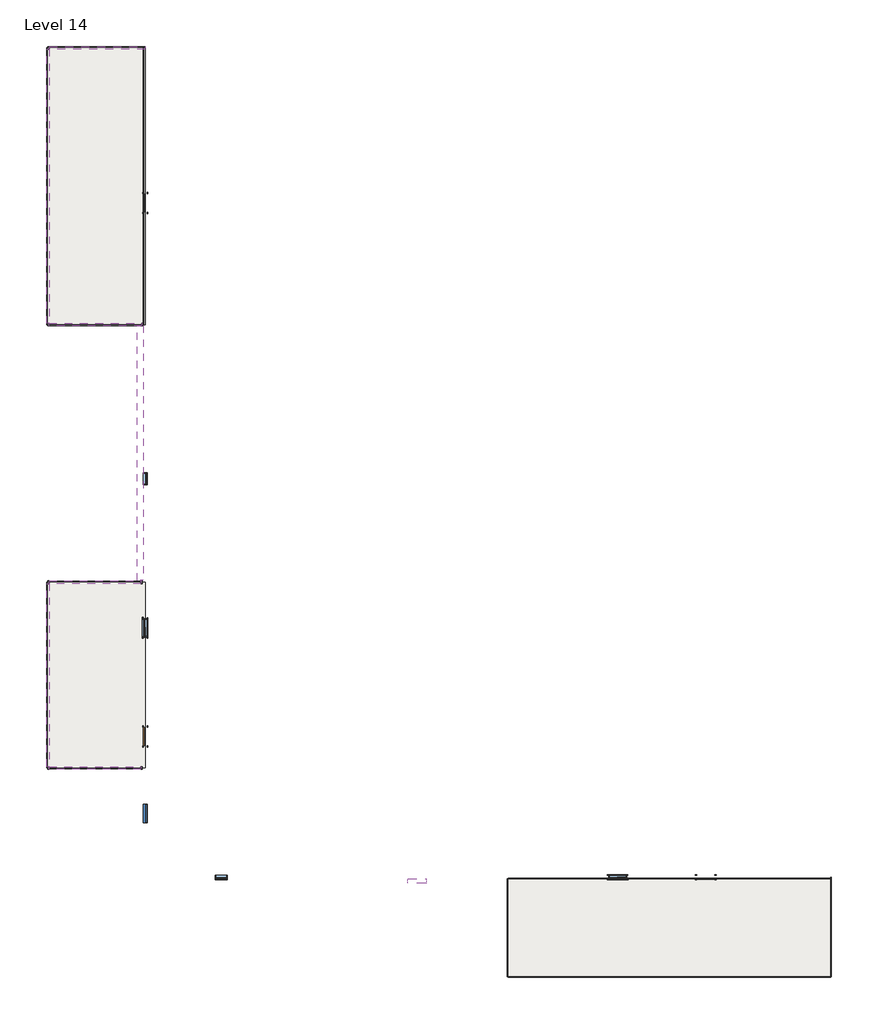
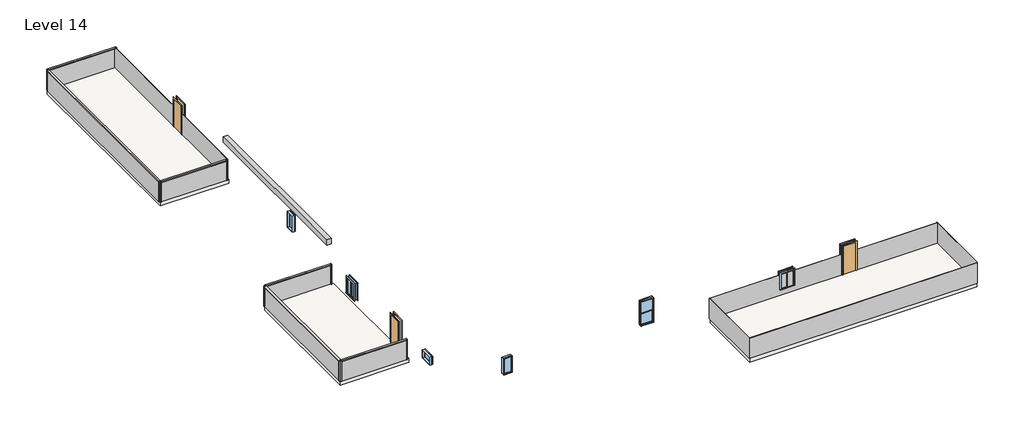
# One storey: 17 members, 11 plates, 6 windows, 3 doors, 3 slabs, 1 proxy.
"""IFC4 building model written with IfcOpenShell, lengths in millimetres."""

from ifc_helpers import new_model, si_unit, frame, origin, place, context, project, spatial, polyline, outline, extrude, transform, mapped, element, save
from components import generic_models_16_generic_models_16_858d129d, door_54dd4da4, door_719f80de, member_a0ba9e48, member_4491d118, member_315671ef, member_43964152, member_8787ee90, member_2afbfae4, system_panel_glazed_dbf8c7ac, system_panel_glazed_64af9de3, system_panel_glazed_abcfc967, system_panel_glazed_48350550, system_panel_glazed_82bc3a22, system_panel_glazed_a411ffd8, system_panel_glazed_b08a8197, system_panel_glazed_fce9463a, system_panel_glazed_627c678d, window_f274a882, window_80bd9af0, window_57c3ee1c, window_78885257, window_54100e87

model = new_model("IFC4")

# Units and contexts
model_context = context("Model", 3, world=origin())
ifc_project = project(units=[si_unit("LENGTHUNIT", "METRE", prefix="MILLI")], contexts=[model_context])

# Site, building, storey
site = spatial("IfcSite", under=ifc_project)
building = spatial("IfcBuilding", under=site)
storey = spatial("IfcBuildingStorey", under=building, Name="Level 14", Elevation=23164.8)

# Proxy
placement = place(None, origin())
generic_models_16_generic_models_16_shape = generic_models_16_generic_models_16_858d129d(model_context)
element("IfcBuildingElementProxy", 1, Name="Generic Models 16 : Generic Models 16", ObjectType="Generic Models 16 : Generic Models 16", at=placement, inside=storey, context=model_context, shape_type="MappedRepresentation", body=[
    mapped(generic_models_16_generic_models_16_shape, transform((0.0, 0.0, 0.0), x_axis=(1.0, 0.0, 0.0), y_axis=(0.0, 1.0, 0.0), z_axis=(0.0, 0.0, 1.0))),
])

# Doors
door_shape = door_54dd4da4(model_context)
element("IfcDoor", 2, ObjectType="Single-Flush : 36\" x 84\"", at=placement, inside=storey, context=model_context, shape_type="MappedRepresentation", body=[
    mapped(door_shape, transform((-15175.038074, 13037.8014639, 23164.8), x_axis=(0.0, 1.0, 0.0), y_axis=(-1.0, 0.0, 0.0), z_axis=(0.0, 0.0, 1.0))),
])
element("IfcDoor", 3, ObjectType="Single-Flush : 36\" x 84\"", at=placement, inside=storey, context=model_context, shape_type="MappedRepresentation", body=[
    mapped(door_shape, transform((-15175.038074, -13700.1915889, 23164.8), x_axis=(0.0, 1.0, 0.0), y_axis=(-1.0, 0.0, 0.0), z_axis=(0.0, 0.0, 1.0))),
])
door_2_shape = door_719f80de(model_context)
element("IfcDoor", 4, ObjectType="Single-Flush : 36\" x 84\"", at=placement, inside=storey, context=model_context, shape_type="MappedRepresentation", body=[
    mapped(door_2_shape, transform((12917.361926, -20744.1985361, 23164.8), x_axis=(1.0, 0.0, 0.0), y_axis=(0.0, 1.0, 0.0), z_axis=(0.0, 0.0, 1.0))),
])

# Members
member_shape = member_a0ba9e48(model_context)
element("IfcMember", 5, ObjectType="Rectangular Mullion : 2.5\" x 5\" rectangular", at=placement, inside=storey, context=model_context, shape_type="MappedRepresentation", body=[
    mapped(member_shape, transform((-15175.038074, 20810.2014639, 24688.8), x_axis=(0.0, 0.0, 1.0), y_axis=(0.0, -1.0, 0.0), z_axis=(1.0, 0.0, 0.0))),
])
member_2_shape = member_4491d118(model_context)
element("IfcMember", 6, ObjectType="Rectangular Mullion : 2.5\" x 5\" rectangular", at=placement, inside=storey, context=model_context, shape_type="MappedRepresentation", body=[
    mapped(member_2_shape, transform((-20051.838074, 6941.8014639, 23164.8), x_axis=(-1.0, 0.0, 0.0), y_axis=(0.0, 1.0, 0.0), z_axis=(0.0, 0.0, -1.0))),
])
element("IfcMember", 7, ObjectType="Rectangular Mullion : 2.5\" x 5\" rectangular", at=placement, inside=storey, context=model_context, shape_type="MappedRepresentation", body=[
    mapped(member_2_shape, transform((-20051.838074, 20810.2014639, 23164.8), x_axis=(0.0, 1.0, 0.0), y_axis=(1.0, 0.0, 0.0), z_axis=(0.0, 0.0, -1.0))),
])
element("IfcMember", 8, ObjectType="Rectangular Mullion : 2.5\" x 5\" rectangular", at=placement, inside=storey, context=model_context, shape_type="MappedRepresentation", body=[
    mapped(member_2_shape, transform((-20051.838074, -15263.2213044, 23164.8), x_axis=(-1.0, 0.0, 0.0), y_axis=(0.0, 1.0, 0.0), z_axis=(0.0, 0.0, -1.0))),
])
element("IfcMember", 9, ObjectType="Rectangular Mullion : 2.5\" x 5\" rectangular", at=placement, inside=storey, context=model_context, shape_type="MappedRepresentation", body=[
    mapped(member_2_shape, transform((-20051.838074, -5966.8213044, 23164.8), x_axis=(0.0, 1.0, 0.0), y_axis=(1.0, 0.0, 0.0), z_axis=(0.0, 0.0, -1.0))),
])
element("IfcMember", 10, ObjectType="Rectangular Mullion : 2.5\" x 5\" rectangular", at=placement, inside=storey, context=model_context, shape_type="MappedRepresentation", body=[
    mapped(member_2_shape, transform((-15319.7124518, -5966.8213044, 23164.8), x_axis=(1.0, 0.0, 0.0), y_axis=(0.0, -1.0, 0.0), z_axis=(0.0, 0.0, -1.0))),
])
element("IfcMember", 11, ObjectType="Rectangular Mullion : 2.5\" x 5\" rectangular", at=placement, inside=storey, context=model_context, shape_type="MappedRepresentation", body=[
    mapped(member_2_shape, transform((-20051.838074, 6941.8014639, 24688.8), x_axis=(0.0, -1.0, 0.0), y_axis=(1.0, 0.0, 0.0), z_axis=(0.0, 0.0, 1.0))),
])
element("IfcMember", 12, ObjectType="Rectangular Mullion : 2.5\" x 5\" rectangular", at=placement, inside=storey, context=model_context, shape_type="MappedRepresentation", body=[
    mapped(member_2_shape, transform((-15282.7172704, 6941.8014639, 24688.8), x_axis=(1.0, 0.0, 0.0), y_axis=(0.0, 1.0, 0.0), z_axis=(0.0, 0.0, 1.0))),
])
element("IfcMember", 13, ObjectType="Rectangular Mullion : 2.5\" x 5\" rectangular", at=placement, inside=storey, context=model_context, shape_type="MappedRepresentation", body=[
    mapped(member_2_shape, transform((-20051.838074, 20810.2014639, 24688.8), x_axis=(-1.0, 0.0, 0.0), y_axis=(0.0, -1.0, 0.0), z_axis=(0.0, 0.0, 1.0))),
])
element("IfcMember", 14, ObjectType="Rectangular Mullion : 2.5\" x 5\" rectangular", at=placement, inside=storey, context=model_context, shape_type="MappedRepresentation", body=[
    mapped(member_2_shape, transform((-20051.838074, -15263.2213044, 24688.8), x_axis=(0.0, -1.0, 0.0), y_axis=(1.0, 0.0, 0.0), z_axis=(0.0, 0.0, 1.0))),
])
element("IfcMember", 15, ObjectType="Rectangular Mullion : 2.5\" x 5\" rectangular", at=placement, inside=storey, context=model_context, shape_type="MappedRepresentation", body=[
    mapped(member_2_shape, transform((-15319.7124518, -15263.2213044, 24688.8), x_axis=(1.0, 0.0, 0.0), y_axis=(0.0, 1.0, 0.0), z_axis=(0.0, 0.0, 1.0))),
])
element("IfcMember", 16, ObjectType="Rectangular Mullion : 2.5\" x 5\" rectangular", at=placement, inside=storey, context=model_context, shape_type="MappedRepresentation", body=[
    mapped(member_2_shape, transform((-20051.838074, -5966.8213044, 24688.8), x_axis=(-1.0, 0.0, 0.0), y_axis=(0.0, -1.0, 0.0), z_axis=(0.0, 0.0, 1.0))),
])
member_3_shape = member_315671ef(model_context)
element("IfcMember", 17, ObjectType="Rectangular Mullion : 2.5\" x 5\" rectangular", at=placement, inside=storey, context=model_context, shape_type="MappedRepresentation", body=[
    mapped(member_3_shape, transform((-20051.838074, 20746.7014639, 24688.8), x_axis=(0.0, 0.0, 1.0), y_axis=(1.0, 0.0, 0.0), z_axis=(0.0, 1.0, 0.0))),
])
member_4_shape = member_43964152(model_context)
element("IfcMember", 18, ObjectType="Rectangular Mullion : 2.5\" x 5\" rectangular", at=placement, inside=storey, context=model_context, shape_type="MappedRepresentation", body=[
    mapped(member_4_shape, transform((-19988.338074, 6941.8014639, 24688.8), x_axis=(0.0, 0.0, 1.0), y_axis=(0.0, 1.0, 0.0), z_axis=(-1.0, 0.0, 0.0))),
])
member_5_shape = member_8787ee90(model_context)
element("IfcMember", 19, ObjectType="Rectangular Mullion : 2.5\" x 5\" rectangular", at=placement, inside=storey, context=model_context, shape_type="MappedRepresentation", body=[
    mapped(member_5_shape, transform((-20051.838074, -6030.3213044, 24688.8), x_axis=(0.0, 0.0, 1.0), y_axis=(1.0, 0.0, 0.0), z_axis=(0.0, 1.0, 0.0))),
])
member_6_shape = member_2afbfae4(model_context)
element("IfcMember", 20, ObjectType="Rectangular Mullion : 2.5\" x 5\" rectangular", at=placement, inside=storey, context=model_context, shape_type="MappedRepresentation", body=[
    mapped(member_6_shape, transform((-19988.338074, -15263.2213044, 24688.8), x_axis=(0.0, 0.0, 1.0), y_axis=(0.0, 1.0, 0.0), z_axis=(-1.0, 0.0, 0.0))),
])
element("IfcMember", 21, ObjectType="Rectangular Mullion : 2.5\" x 5\" rectangular", at=placement, inside=storey, context=model_context, shape_type="MappedRepresentation", body=[
    mapped(member_6_shape, transform((-15383.2124518, -5966.8213044, 24688.8), x_axis=(0.0, 0.0, 1.0), y_axis=(0.0, -1.0, 0.0), z_axis=(1.0, 0.0, 0.0))),
])

# Plates
system_panel_glazed_shape = system_panel_glazed_dbf8c7ac(model_context)
element("IfcPlate", 22, ObjectType="System Panel : Glazed", at=placement, inside=storey, context=model_context, shape_type="MappedRepresentation", body=[
    mapped(system_panel_glazed_shape, transform((11088.561926, -20845.7985361, 23164.8), x_axis=(1.0, 0.0, 0.0), y_axis=(0.0, 1.0, 0.0), z_axis=(0.0, 0.0, 1.0))),
])
element("IfcPlate", 23, ObjectType="System Panel : Glazed", at=placement, inside=storey, context=model_context, shape_type="MappedRepresentation", body=[
    mapped(system_panel_glazed_shape, transform((11088.561926, -25722.5985361, 23164.8), x_axis=(-1.0, 0.0, 0.0), y_axis=(0.0, -1.0, 0.0), z_axis=(0.0, 0.0, 1.0))),
])
system_panel_glazed_2_shape = system_panel_glazed_64af9de3(model_context)
element("IfcPlate", 24, ObjectType="System Panel : Glazed", at=placement, inside=storey, context=model_context, shape_type="MappedRepresentation", body=[
    mapped(system_panel_glazed_2_shape, transform((19165.761926, -23233.3985361, 23164.8), x_axis=(0.0, -1.0, 0.0), y_axis=(1.0, 0.0, 0.0), z_axis=(0.0, 0.0, 1.0))),
])
system_panel_glazed_3_shape = system_panel_glazed_abcfc967(model_context)
element("IfcPlate", 25, ObjectType="System Panel : Glazed", at=placement, inside=storey, context=model_context, shape_type="MappedRepresentation", body=[
    mapped(system_panel_glazed_3_shape, transform((3011.361926, -23273.4060583, 23164.8), x_axis=(0.0, 1.0, 0.0), y_axis=(-1.0, 0.0, 0.0), z_axis=(0.0, 0.0, 1.0))),
])
system_panel_glazed_4_shape = system_panel_glazed_48350550(model_context)
element("IfcPlate", 26, ObjectType="System Panel : Glazed", at=placement, inside=storey, context=model_context, shape_type="MappedRepresentation", body=[
    mapped(system_panel_glazed_4_shape, transform((-15282.7172704, 13876.0014639, 23164.8), x_axis=(0.0, -1.0, 0.0), y_axis=(1.0, 0.0, 0.0), z_axis=(0.0, 0.0, 1.0))),
])
system_panel_glazed_5_shape = system_panel_glazed_82bc3a22(model_context)
element("IfcPlate", 27, ObjectType="System Panel : Glazed", at=placement, inside=storey, context=model_context, shape_type="MappedRepresentation", body=[
    mapped(system_panel_glazed_5_shape, transform((-17581.688074, 20810.2014639, 23164.8), x_axis=(1.0, 0.0, 0.0), y_axis=(0.0, 1.0, 0.0), z_axis=(0.0, 0.0, 1.0))),
])
system_panel_glazed_6_shape = system_panel_glazed_a411ffd8(model_context)
element("IfcPlate", 28, ObjectType="System Panel : Glazed", at=placement, inside=storey, context=model_context, shape_type="MappedRepresentation", body=[
    mapped(system_panel_glazed_6_shape, transform((-20051.838074, 13876.0014639, 23164.8), x_axis=(0.0, 1.0, 0.0), y_axis=(-1.0, 0.0, 0.0), z_axis=(0.0, 0.0, 1.0))),
])
system_panel_glazed_7_shape = system_panel_glazed_b08a8197(model_context)
element("IfcPlate", 29, ObjectType="System Panel : Glazed", at=placement, inside=storey, context=model_context, shape_type="MappedRepresentation", body=[
    mapped(system_panel_glazed_7_shape, transform((-17667.2776722, 6941.8014639, 23164.8), x_axis=(-1.0, 0.0, 0.0), y_axis=(0.0, -1.0, 0.0), z_axis=(0.0, 0.0, 1.0))),
])
system_panel_glazed_8_shape = system_panel_glazed_fce9463a(model_context)
element("IfcPlate", 30, ObjectType="System Panel : Glazed", at=placement, inside=storey, context=model_context, shape_type="MappedRepresentation", body=[
    mapped(system_panel_glazed_8_shape, transform((-20051.838074, -10615.0213044, 23164.8), x_axis=(0.0, 1.0, 0.0), y_axis=(-1.0, 0.0, 0.0), z_axis=(0.0, 0.0, 1.0))),
])
system_panel_glazed_9_shape = system_panel_glazed_627c678d(model_context)
element("IfcPlate", 31, ObjectType="System Panel : Glazed", at=placement, inside=storey, context=model_context, shape_type="MappedRepresentation", body=[
    mapped(system_panel_glazed_9_shape, transform((-17685.7752629, -5966.8213044, 23164.8), x_axis=(1.0, 0.0, 0.0), y_axis=(0.0, 1.0, 0.0), z_axis=(0.0, 0.0, 1.0))),
])
element("IfcPlate", 32, ObjectType="System Panel : Glazed", at=placement, inside=storey, context=model_context, shape_type="MappedRepresentation", body=[
    mapped(system_panel_glazed_9_shape, transform((-17685.7752629, -15263.2213044, 23164.8), x_axis=(-1.0, 0.0, 0.0), y_axis=(0.0, -1.0, 0.0), z_axis=(0.0, 0.0, 1.0))),
])

# Slabs
element("IfcSlab", 33, ObjectType="Generic - 12\"", at=placement, inside=storey, context=model_context, shape_type="SweptSolid", body=[
    extrude(outline(polyline([(3011.361926, -20845.7985361), (19165.761926, -20845.7985361), (19165.761926, -25722.5985361), (3011.361926, -25722.5985361), (3011.361926, -20845.7985361)])), frame((0.0, 0.0, 22860.0), z_axis=(0.0, 0.0, 1.0), x_axis=(1.0, 0.0, 0.0)), (0.0, 0.0, 1.0), 304.8),
])
element("IfcSlab", 34, ObjectType="Generic - 12\"", at=placement, inside=storey, context=model_context, shape_type="SweptSolid", body=[
    extrude(outline(polyline([(-20051.838074, -15263.2213044), (-20051.838074, -5966.8213044), (-15175.038074, -5966.8213044), (-15175.038074, -15263.2213044), (-20051.838074, -15263.2213044)])), frame((0.0, 0.0, 22860.0), z_axis=(0.0, 0.0, 1.0), x_axis=(1.0, 0.0, 0.0)), (0.0, 0.0, 1.0), 304.8),
])
element("IfcSlab", 35, ObjectType="Generic - 12\"", at=placement, inside=storey, context=model_context, shape_type="SweptSolid", body=[
    extrude(outline(polyline([(-20051.838074, 20810.2014639), (-15175.038074, 20810.2014639), (-15175.038074, 6941.8014639), (-20051.838074, 6941.8014639), (-20051.838074, 20810.2014639)])), frame((0.0, 0.0, 22860.0), z_axis=(0.0, 0.0, 1.0), x_axis=(1.0, 0.0, 0.0)), (0.0, 0.0, 1.0), 304.8),
])

# Windows
window_shape = window_f274a882(model_context)
element("IfcWindow", 36, ObjectType="Double Hung : 36\" x 72\"", at=placement, inside=storey, context=model_context, shape_type="MappedRepresentation", body=[
    mapped(window_shape, transform((-1560.638074, -20921.9985361, 24167.4535848), x_axis=(-1.0, 0.0, 0.0), y_axis=(0.0, -1.0, 0.0), z_axis=(0.0, 0.0, 1.0))),
])
window_2_shape = window_80bd9af0(model_context)
element("IfcWindow", 37, ObjectType="Fixed : 24\" x 48\"", at=placement, inside=storey, context=model_context, shape_type="MappedRepresentation", body=[
    mapped(window_2_shape, transform((-15175.038074, -823.3213044, 23164.8), x_axis=(0.0, -1.0, 0.0), y_axis=(1.0, 0.0, 0.0), z_axis=(0.0, 0.0, 1.0))),
])
window_3_shape = window_57c3ee1c(model_context)
element("IfcWindow", 38, ObjectType="Fixed : 36\" x 24\"", at=placement, inside=storey, context=model_context, shape_type="MappedRepresentation", body=[
    mapped(window_3_shape, transform((-15175.038074, -17587.3213044, 23429.0717638), x_axis=(0.0, -1.0, 0.0), y_axis=(1.0, 0.0, 0.0), z_axis=(0.0, 0.0, 1.0))),
])
window_4_shape = window_78885257(model_context)
element("IfcWindow", 39, ObjectType="Instance - Fixed : 24\" x 48\"", at=placement, inside=storey, context=model_context, shape_type="MappedRepresentation", body=[
    mapped(window_4_shape, transform((-11403.138074, -20744.1985361, 23164.8), x_axis=(-1.0, 0.0, 0.0), y_axis=(0.0, -1.0, 0.0), z_axis=(0.0, 0.0, 1.0))),
])
window_5_shape = window_54100e87(model_context)
element("IfcWindow", 40, ObjectType="Slider with Trim : 36\" x 48\"", at=placement, inside=storey, context=model_context, shape_type="MappedRepresentation", body=[
    mapped(window_5_shape, transform((8497.761926, -20744.1985361, 22673.1129205), x_axis=(-1.0, 0.0, 0.0), y_axis=(0.0, -1.0, 0.0), z_axis=(0.0, 0.0, 1.0))),
])
element("IfcWindow", 41, ObjectType="Slider with Trim : 36\" x 48\"", at=placement, inside=storey, context=model_context, shape_type="MappedRepresentation", body=[
    mapped(window_5_shape, transform((-15175.038074, -8252.8213044, 22661.2201055), x_axis=(0.0, 1.0, 0.0), y_axis=(-1.0, 0.0, 0.0), z_axis=(0.0, 0.0, 1.0))),
])

save(model, "model.ifc")

# Revit data of these elements
# Type "Single-Flush : 36\" x 84\""
#   Type Mark = "1"
#   Construction Type Id = "MDOOR"
#   Assembly Code = "C1020"
#   Analytic Construction = "Metal"
#   Thickness = 0' - 2"
#   Heat Transfer Coefficient (U) = 0.651978 BTU/(h·ft²·°F)
#   Height = 7' - 0"
#   Trim Projection Ext = 0' - 1"
#   Trim Projection Int = 0' - 1"
#   Trim Width = 0' - 3"
#   Width = 3' - 0"
#   Define Thermal Properties by = 1
#   Door Material = Door - Panel
#   Frame Material = Door - Frame
#   Visual Light Transmittance = 0
#   Solar Heat Gain Coefficient = 0
#   Function = (empty or 0)
#   Wall Closure = (empty or 0)
# Type "Rectangular Mullion : 2.5\" x 5\" rectangular"
#   built-in parameter 1007304 = 0.416667 (stored number, unit not read)
#   built-in parameter 1007301 = 0.104167 (stored number, unit not read)
#   built-in parameter 1007300 = 0.104167 (stored number, unit not read)
# Type "System Panel : Glazed"
#   Construction Type Id = "GSP4R"
#   Analytic Construction = "1/8 in Pilkington single glazing"
#   Visual Light Transmittance = 0.9
#   Solar Heat Gain Coefficient = 0.86
#   Heat Transfer Coefficient (U) = 1.18115 BTU/(h·ft²·°F)
# Type "Generic - 12\""
#   Assembly Code = "B1010"
#   Function = 0
#   Layers, outside or top first: 1' - 0" no material (function 1)
# Type "Double Hung : 36\" x 72\""
#   Type Mark = "18"
#   Construction Type Id = "GSP4R"
#   Assembly Code = "B2020100"
#   Analytic Construction = "1/8 in Pilkington single glazing"
#   Visual Light Transmittance = 0.9
#   Solar Heat Gain Coefficient = 0.78
#   Heat Transfer Coefficient (U) = 0.6496 BTU/(h·ft²·°F)
#   Height = 6' - 0"
#   Default Sill Height = 1' - 0"
#   Width = 3' - 0"
#   Window Inset = 0' - 0 3/4"
#   Define Thermal Properties by = 1
#   Glass Pane Material = Glass
#   Sash Material = Sash
#   Description = (empty or 0)
#   Wall Closure = (empty or 0)
# Type "Fixed : 24\" x 48\""
#   Type Mark = "2"
#   Construction Type Id = "GSP4R"
#   Assembly Code = "B2020100"
#   Analytic Construction = "1/8 in Pilkington single glazing"
#   Visual Light Transmittance = 0.9
#   Solar Heat Gain Coefficient = 0.78
#   Heat Transfer Coefficient (U) = 0.6496 BTU/(h·ft²·°F)
#   Height = 4' - 0"
#   Default Sill Height = 3' - 0"
#   Width = 2' - 0"
#   Window Inset = 0' - 0 3/4"
#   Define Thermal Properties by = 1
#   Glass Pane Material = Glass
#   Sash Material = Sash
#   Wall Closure = (empty or 0)
# Type "Fixed : 36\" x 24\""
#   Type Mark = "8"
#   Construction Type Id = "GSP4R"
#   Assembly Code = "B2020100"
#   Analytic Construction = "1/8 in Pilkington single glazing"
#   Visual Light Transmittance = 0.9
#   Solar Heat Gain Coefficient = 0.78
#   Heat Transfer Coefficient (U) = 0.6496 BTU/(h·ft²·°F)
#   Height = 2' - 0"
#   Default Sill Height = 3' - 0"
#   Width = 3' - 0"
#   Window Inset = 0' - 0 3/4"
#   Define Thermal Properties by = 1
#   Glass Pane Material = Glass
#   Sash Material = Sash
#   Wall Closure = (empty or 0)
# Type "Instance - Fixed : 24\" x 48\""
#   Type Mark = "19"
#   Construction Type Id = "GSP4R"
#   Assembly Code = "B2020100"
#   Analytic Construction = "1/8 in Pilkington single glazing"
#   Visual Light Transmittance = 0.9
#   Thermal Resistance (R) = 0.8466 (h·ft²·°F)/BTU
#   Solar Heat Gain Coefficient = 0.86
#   Heat Transfer Coefficient (U) = 1.1812 BTU/(h·ft²·°F)
#   Height [instance default] = 4' - 0"
#   Default Sill Height = 3' - 0"
#   Width [instance default] = 2' - 0"
#   Window Inset = 0' - 0 3/4"
#   Define Thermal Properties by = 1
#   Glass Pane Material = Glass
#   Sash Material = Sash
#   Wall Closure = (empty or 0)
# Type "Slider with Trim : 36\" x 48\""
#   Type Mark = "22"
#   Construction Type Id = "GSP4R"
#   Assembly Code = "B2020100"
#   Analytic Construction = "1/8 in Pilkington single glazing"
#   Visual Light Transmittance = 0.9
#   Solar Heat Gain Coefficient = 0.78
#   Heat Transfer Coefficient (U) = 0.6496 BTU/(h·ft²·°F)
#   Height = 4' - 0"
#   Default Sill Height = 3' - 0"
#   Trim Projection - Ext. = 0' - 0 3/4"
#   Trim Projection - Int. = 0' - 0 3/4"
#   Trim Width - Exterior = 0' - 3 1/2"
#   Trim Width - Interior = 0' - 3 1/2"
#   Width = 3' - 0"
#   Window Inset = 0' - 0 3/4"
#   Define Thermal Properties by = 1
#   Glass Pane Material = Glass
#   Sash Material = Sash
#   Trim Exterior Material = Trim
#   Trim Interior Material = Trim
#   Wall Closure = (empty or 0)
# Element 1 (IfcBuildingElementProxy, "Generic Models 16 : Generic Models 16")
#   Phase Created = New Construction
# Elements 2, 3, 4 (IfcDoor, "Single-Flush : 36\" x 84\"")
#   Phase Created = New Construction
#   Materials on its faces: "Door - Frame", "Door - Panel"
# Elements 5, 6, 7, 8, 9, 10, 11, 12, 13, 14, 15, 16, 17, 18, 19, 20, 21 (IfcMember, "Rectangular Mullion : 2.5\" x 5\" rectangular")
#   Phase Created = New Construction
#   Materials on its faces: "Aluminum"
# Elements 22, 23, 24, 25, 26, 27, 28, 29, 30, 31, 32 (IfcPlate, "System Panel : Glazed")
#   Phase Created = New Construction
#   Materials on its faces: "Glass"
# Elements 33, 34, 35 (IfcSlab, "Generic - 12\"")
#   built-in parameter 1001955 = 3.14159 (stored number, unit not read)
#   Height Offset From Level = 0' - 0"
#   Phase Created = New Construction
#   Materials on its faces: "Default Floor"
# Element 36 (IfcWindow, "Double Hung : 36\" x 72\"")
#   Mark = "4"
#   Phase Created = New Construction
#   Materials on its faces: "Sash", "Glass"
# Element 37 (IfcWindow, "Fixed : 24\" x 48\"")
#   Mark = "49"
#   Phase Created = New Construction
#   Materials on its faces: "Sash", "Glass"
# Element 38 (IfcWindow, "Fixed : 36\" x 24\"")
#   Mark = "71"
#   Phase Created = New Construction
#   Materials on its faces: "Sash", "Glass"
# Element 39 (IfcWindow, "Instance - Fixed : 24\" x 48\"")
#   Mark = "17"
#   Width = 2' - 0"
#   Height = 4' - 0"
#   Phase Created = New Construction
#   Materials on its faces: "Sash", "Glass"
# Element 40 (IfcWindow, "Slider with Trim : 36\" x 48\"")
#   Mark = "27"
#   Phase Created = New Construction
#   Materials on its faces: "Sash", "Trim", "Glass"
# Element 41 (IfcWindow, "Slider with Trim : 36\" x 48\"")
#   Mark = "38"
#   Phase Created = New Construction
#   Materials on its faces: "Sash", "Trim", "Glass"
# Materials
#   "Door - Panel": class "Wood", colour RGB 210 159 95, transparency 0
#   "Door - Frame": colour RGB 118 70 51, transparency 0
#   "Glass": class "Glass", colour RGB 0 128 192, transparency 0.75, Description = "Soda Lime Glass", Cost = 0
#   "Sash": class "Wood", colour RGB 224 178 126, transparency 0
#   "Trim": class "Wood", colour RGB 224 178 126, transparency 0
#   "Aluminum": class "Metal", colour RGB 247 247 247, transparency 0, Description = "Aluminum 6061", Cost = 0
#   "Default Floor": colour RGB 128 128 128, transparency 0
